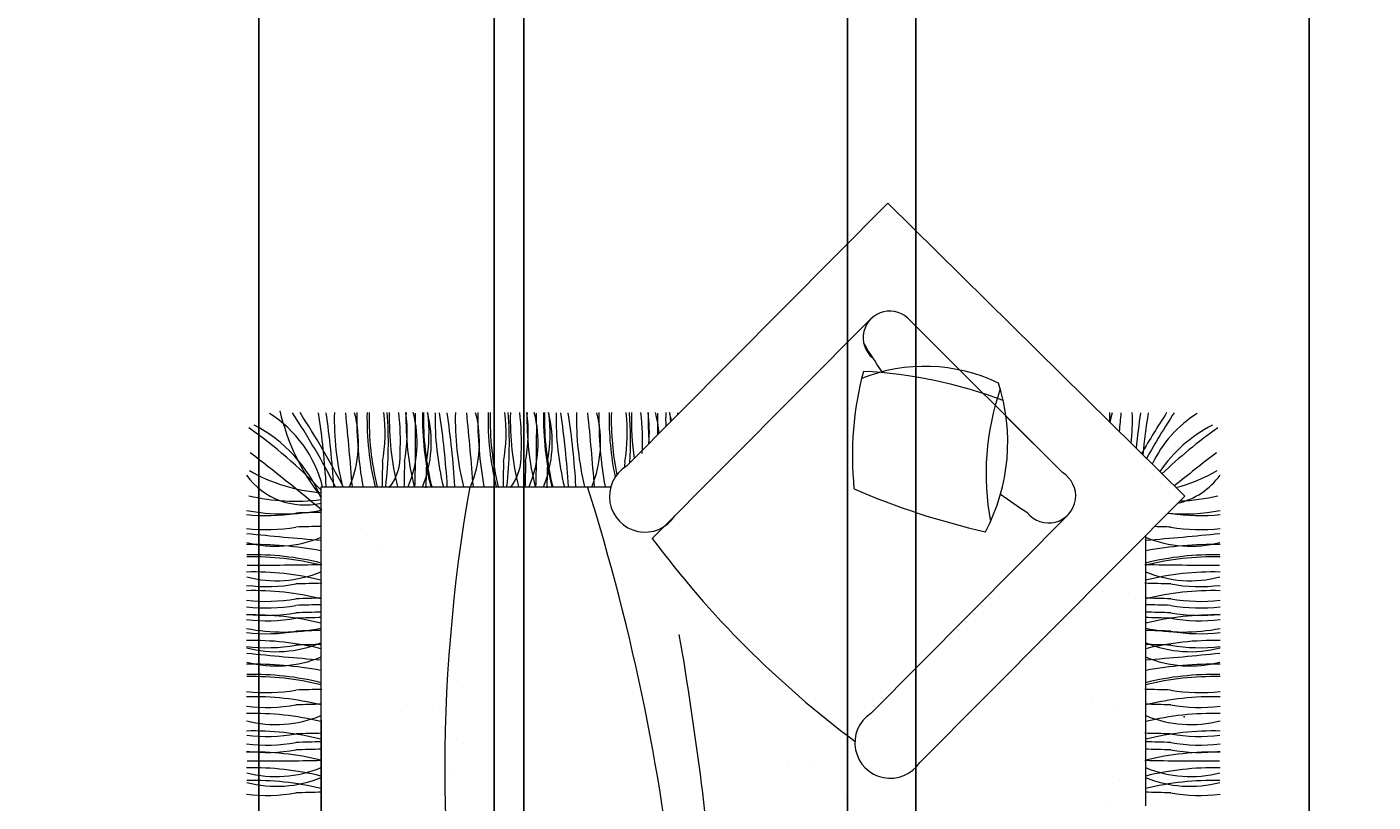
# Model space of a CAD drawing. Units: inches. Extents: x 503 to 1084, y -605 to 132.
# Tile 10 of 14: x 882 to 974, y -230 to -177. Entities that reach past the tile are written whole.
import ezdxf

# ---------------------------------------------------------------- set-up
doc = ezdxf.new("R2010")
doc.units = ezdxf.units.IN
doc.header["$MEASUREMENT"] = 0
doc.layers.add('A-ANNO-DIMS', color=7, linetype='Continuous', lineweight=18)
doc.layers.add('furniture', color=50, linetype='Continuous', lineweight=13, transparency=0.8)
doc.styles.get("Standard").update_dxf_attribs({"font": 'arial.ttf'})
doc.dimstyles.get("Standard").update_dxf_attribs({"dimtxt": 0.18, "dimasz": 0.18, "dimexe": 0.18, "dimexo": 0.0625, "dimgap": 0.09, "dimtad": 0, "dimtih": 1, "dimtoh": 1, "dimdec": 1, "dimzin": 0, "dimdsep": 46, "dimlunit": 4, "dimtxsty": 'Standard', "dimcen": 0.09, "dimadec": 0, "dimazin": 0, "dimtfac": 1, "dimtdec": 1, "dimtofl": 0, "dimtmove": 0, "dimatfit": 3, "dimfxl": 1, "dimtolj": 1, "dimtzin": 0, "dimarcsym": 0})

# ---------------------------------------------------------------- blocks, each defined once
blk = doc.blocks.new('CUSHION-SCATTER')
for centre, radius, start, end in [((-0.355, -5.979), 11.599, 64.45006, 111.76991), ((17.467, -0.489), 22.747, 165.30685, 185.5663), ((-5.995, -25.402), 30.717, 69.08153, 87.27682), ((-7.72, 0.481), 12.999, 332.0126, 17.9429), ((21.395, -1.669), 17.594, 160.90051, 190.65125), ((14.361, 41.881), 48.668, 246.33709, 257.41765)]:
    blk.add_arc(centre, radius, start, end)
blk = doc.blocks.new('*D45')
at = {"layer": 'A-ANNO-DIMS', "color": 0, "lineweight": -2, "transparency": 16777216}
for p, q in [((844.089, -354.753), (844.089, 43.514)), ((844.269, 43.334), (879.759, 43.334)), ((915.909, 43.334), (880.418, 43.334)), ((916.089, -354.753), (916.089, 43.514))]:
    blk.add_line(p, q, dxfattribs=at)
at = {"layer": 'A-ANNO-DIMS', "color": 0, "transparency": 16777216}
for points in [[(844.269, 43.364), (844.269, 43.304), (844.089, 43.334)], [(915.909, 43.364), (915.909, 43.304), (916.089, 43.334)]]:
    blk.add_solid(points, dxfattribs=at)
at = {"layer": 'Defpoints', "color": 0, "transparency": 16777216}
for p in [(916.089, 43.334), (844.089, -354.816), (916.089, -354.816)]:
    blk.add_point(p, dxfattribs=at)
at = {"layer": 'A-ANNO-DIMS', "color": 0, "transparency": 16777216, "insert": (880.089, 43.334), "char_height": 0.18, "attachment_point": 5}
blk.add_mtext('\\A1;6\'-0"', dxfattribs=at)
blk = doc.blocks.new('*D64')
at = {"layer": 'A-ANNO-DIMS', "color": 0, "lineweight": -2, "transparency": 16777216}
for p, q in [((938.089, -162.878), (938.089, -583.146)), ((977.089, -162.878), (977.089, -583.146)), ((938.269, -582.966), (957.26, -582.966)), ((976.909, -582.966), (957.918, -582.966))]:
    blk.add_line(p, q, dxfattribs=at)
at = {"layer": 'A-ANNO-DIMS', "color": 0, "transparency": 16777216}
for points in [[(938.269, -582.936), (938.269, -582.996), (938.089, -582.966)], [(976.909, -582.936), (976.909, -582.996), (977.089, -582.966)]]:
    blk.add_solid(points, dxfattribs=at)
at = {"layer": 'Defpoints', "color": 0, "transparency": 16777216}
for p in [(938.089, -162.816), (977.089, -162.816), (977.089, -582.966)]:
    blk.add_point(p, dxfattribs=at)
at = {"layer": 'A-ANNO-DIMS', "color": 0, "transparency": 16777216, "insert": (957.589, -582.966), "char_height": 0.18, "attachment_point": 5}
blk.add_mtext('\\A1;3\'-3"', dxfattribs=at)
blk = doc.blocks.new('*D65')
at = {"layer": 'A-ANNO-DIMS', "color": 0, "lineweight": -2, "transparency": 16777216}
for p, q in [((898.089, -162.878), (898.089, -583.146)), ((914.089, -162.878), (914.089, -583.146)), ((898.269, -582.966), (905.768, -582.966)), ((913.909, -582.966), (906.409, -582.966))]:
    blk.add_line(p, q, dxfattribs=at)
at = {"layer": 'A-ANNO-DIMS', "color": 0, "transparency": 16777216}
for points in [[(898.269, -582.936), (898.269, -582.996), (898.089, -582.966)], [(913.909, -582.936), (913.909, -582.996), (914.089, -582.966)]]:
    blk.add_solid(points, dxfattribs=at)
at = {"layer": 'Defpoints', "color": 0, "transparency": 16777216}
for p in [(898.089, -162.816), (914.089, -162.816), (914.089, -582.966)]:
    blk.add_point(p, dxfattribs=at)
at = {"layer": 'A-ANNO-DIMS', "color": 0, "transparency": 16777216, "insert": (906.089, -582.966), "char_height": 0.18, "attachment_point": 5}
blk.add_mtext('\\A1;1\'-4"', dxfattribs=at)
blk = doc.blocks.new('*D71')
at = {"layer": 'A-ANNO-DIMS', "color": 0, "lineweight": -2, "transparency": 16777216}
for p, q in [((942.746, -236.149), (942.746, 43.514)), ((942.926, 43.334), (955.566, 43.334)), ((969.287, 43.334), (956.647, 43.334)), ((969.467, -235.109), (969.467, 43.514))]:
    blk.add_line(p, q, dxfattribs=at)
at = {"layer": 'A-ANNO-DIMS', "color": 0, "transparency": 16777216}
for points in [[(942.926, 43.364), (942.926, 43.304), (942.746, 43.334)], [(969.287, 43.364), (969.287, 43.304), (969.467, 43.334)]]:
    blk.add_solid(points, dxfattribs=at)
at = {"layer": 'Defpoints', "color": 0, "transparency": 16777216}
for p in [(969.467, 43.334), (969.467, -235.171), (942.746, -236.212)]:
    blk.add_point(p, dxfattribs=at)
at = {"layer": 'A-ANNO-DIMS', "color": 0, "transparency": 16777216, "insert": (956.106, 43.334), "char_height": 0.18, "attachment_point": 5}
blk.add_mtext('\\A1;2\'-2 1/2"', dxfattribs=at)

msp = doc.modelspace()

# ---------------------------------------------------------------- linework, layer by layer
at = {"layer": 'furniture'}
for p, q in [((940.842, -188.826), (923.073, -206.695)), ((961.008, -208.74), (940.842, -188.826)), ((924.828, -211.612), (939.689, -196.679)), ((952.695, -207.138), (942.35, -196.793)), ((945.712, -200.155), (942.35, -196.793)), ((952.695, -207.138), (948.869, -203.312)), ((909.841, -204.939), (909.841, -204.939)), ((909.88, -205.415), (909.88, -205.415)), ((918.065, -204.939), (918.065, -204.939)), ((918.104, -205.415), (918.104, -205.415)), ((902.315, -308.222), (902.315, -208.108)), ((902.315, -208.108), (922.005, -208.108)), ((961.008, -208.74), (943.01, -226.844)), ((900.735, -209.7), (900.735, -209.7)), ((900.735, -209.7), (900.735, -209.7)), ((900.735, -209.7), (900.735, -209.7)), ((953.063, -210.02), (939.67, -223.504)), ((959.933, -209.7), (959.933, -209.7)), ((959.933, -209.7), (959.933, -209.7)), ((959.933, -209.7), (959.933, -209.7)), ((901.032, -210.912), (901.032, -210.912)), ((901.032, -210.912), (901.032, -210.912)), ((901.032, -210.912), (901.032, -210.912)), ((905.046, -210.939), (905.046, -210.939)), ((959.636, -210.912), (959.636, -210.912)), ((959.636, -210.912), (959.636, -210.912)), ((959.636, -210.912), (959.636, -210.912)), ((958.353, -211.41), (958.353, -229.789)), ((906.12, -212.447), (906.12, -212.447)), ((958.875, -213.557), (958.875, -213.557)), ((958.875, -213.557), (958.875, -213.557)), ((955.388, -215.247), (955.388, -215.247)), ((957.16, -215.375), (957.16, -215.375)), ((959.301, -217.841), (959.301, -217.841)), ((958.677, -219.623), (958.677, -219.623)), ((911.581, -221.238), (911.581, -221.238)), ((911.581, -221.238), (911.581, -221.238)), ((908.094, -222.928), (908.094, -222.928)), ((909.866, -223.056), (909.866, -223.056)), ((954.682, -222.776), (954.682, -222.776)), ((956.203, -222.893), (956.203, -222.893)), ((902.315, -223.932), (902.315, -308.222)), ((958.383, -223.668), (958.383, -223.668)), ((961.321, -223.379), (961.321, -223.379)), ((912.007, -225.523), (912.007, -225.523)), ((937.593, -225.079), (937.593, -225.079)), ((937.593, -225.079), (937.593, -225.079)), ((934.106, -226.769), (934.106, -226.769)), ((960.596, -226.163), (960.596, -226.163)), ((911.383, -227.304), (911.383, -227.304)), ((935.878, -226.897), (935.878, -226.897)), ((956.6, -227.987), (956.6, -227.987)), ((960.798, -228.54), (960.798, -228.54)), ((938.019, -229.364), (938.019, -229.364)), ((955.877, -229.481), (955.877, -229.481))]:
    msp.add_line(p, q, dxfattribs=at)
for centre, radius, start, end in [((940.967, -197.957), 1.807, 40.10925, 229.89075), ((969.526, -180.121), 35.395, 211.08667, 214.72696), ((914.057, -199.591), 14.916, 192.95229, 218.0769), ((853.121, -233.97), 56.461, 27.26685, 33.17806), ((853.631, -233.957), 56.461, 27.26685, 33.17806), ((847.93, -211.294), 54.836, 3.36442, 8.62286), ((848.44, -211.281), 54.836, 3.36442, 8.62286), ((922.401, -203.504), 19.184, 178.63307, 193.85735), ((681.204, -225.711), 223.934, 4.51462, 5.80171), ((896.994, -205.077), 7.865, 337.30984, 14.86132), ((930.218, -203.485), 25.474, 179.01954, 190.40392), ((924.623, -203.513), 19.184, 178.63307, 193.85735), ((924.766, -203.513), 19.184, 178.63307, 193.85735), ((895.286, -204.416), 11.387, 349.93491, 6.88295), ((880.977, -205.084), 25.914, 353.37018, 4.50636), ((926.135, -203.508), 19.184, 178.63307, 193.85735), ((889.96, -205.04), 17.75, 357.44348, 6.44133), ((896.783, -204.411), 11.387, 349.93491, 6.88295), ((927.27, -203.499), 19.184, 178.63307, 193.85735), ((900.98, -205.061), 7.865, 337.30984, 14.86132), ((901.945, -205.074), 7.865, 337.30984, 14.86132), ((928.398, -203.511), 19.184, 178.63307, 193.85735), ((928.462, -203.501), 19.184, 178.63307, 193.85735), ((898.269, -204.421), 11.387, 349.93491, 6.88295), ((929.255, -203.519), 19.184, 178.63307, 193.85735), ((856.154, -211.294), 54.836, 3.36442, 8.62286), ((856.664, -211.281), 54.836, 3.36442, 8.62286), ((930.624, -203.504), 19.184, 178.63307, 193.85735), ((689.428, -225.711), 223.934, 4.51462, 5.80171), ((905.218, -205.077), 7.865, 337.30984, 14.86132), ((938.442, -203.485), 25.474, 179.01954, 190.40392), ((932.847, -203.513), 19.184, 178.63307, 193.85735), ((932.99, -203.513), 19.184, 178.63307, 193.85735), ((903.51, -204.416), 11.387, 349.93491, 6.88295), ((889.201, -205.084), 25.914, 353.37018, 4.50636), ((934.359, -203.508), 19.184, 178.63307, 193.85735), ((898.184, -205.04), 17.75, 357.44348, 6.44133), ((905.007, -204.411), 11.387, 349.93491, 6.88295), ((935.494, -203.499), 19.184, 178.63307, 193.85735), ((909.204, -205.061), 7.865, 337.30984, 14.86132), ((910.169, -205.074), 7.865, 337.30984, 14.86132), ((936.622, -203.511), 19.184, 178.63307, 193.85735), ((936.686, -203.501), 19.184, 178.63307, 193.85735), ((906.493, -204.421), 11.387, 349.93491, 6.88295), ((937.479, -203.519), 19.184, 178.63307, 193.85735), ((864.387, -211.294), 54.836, 3.36442, 8.62286), ((864.897, -211.281), 54.836, 3.36442, 8.62286), ((938.857, -203.504), 19.184, 178.63307, 193.85735), ((697.661, -225.711), 223.934, 4.51462, 5.80171), ((913.451, -205.077), 7.865, 337.30984, 14.86132), ((946.675, -203.485), 25.474, 179.01954, 190.40392), ((941.08, -203.513), 19.184, 178.63307, 191.83019), ((941.223, -203.513), 19.184, 178.63307, 191.35191), ((911.743, -204.416), 11.387, 349.93491, 6.88295), ((897.434, -205.084), 25.914, 356.96769, 4.50636), ((942.592, -203.508), 19.184, 178.63307, 187.97978), ((906.417, -205.04), 17.75, 357.44348, 6.44133), ((943.727, -203.499), 19.184, 178.63307, 184.92383), ((913.24, -204.411), 11.387, 356.24526, 6.88295), ((917.437, -205.061), 7.865, 4.27566, 14.86132), ((944.919, -203.501), 19.184, 178.63307, 181.52384), ((918.402, -205.074), 7.865, 10.65917, 14.86132), ((914.725, -204.421), 11.387, 3.81728, 6.88295), ((945.711, -203.519), 19.184, 178.63307, 179.10459), ((930.45, -203.485), 25.474, 359.47531, 0.98046), ((963.674, -205.077), 7.865, 165.13868, 170.07522), ((1179.464, -225.711), 223.934, 174.19829, 174.52363), ((938.268, -203.504), 19.184, 355.05376, 1.36693), ((1012.228, -211.281), 54.836, 171.37714, 173.92031), ((1007.037, -233.957), 56.461, 146.82194, 150.13556), ((1012.738, -211.294), 54.836, 171.37714, 174.38877), ((1007.547, -233.97), 56.461, 146.82194, 150.50261), ((893.328, -212.521), 9.701, 22.11811, 62.69671), ((894.389, -210.105), 8.279, 13.99349, 57.72877), ((744.513, -204.223), 164.233, 358.62796, 0.39341), ((752.737, -204.223), 164.233, 358.62796, 0.39341), ((760.97, -204.223), 164.233, 359.8849, 0.39341), ((966.279, -210.105), 8.279, 122.27123, 154.62744), ((967.34, -212.521), 9.701, 117.30329, 145.70162), ((877.858, -231.706), 33.837, 43.716, 54.68473), ((982.81, -231.706), 33.837, 125.31527, 133.64566), ((802.813, -328.985), 155.386, 50.15682, 52.45592), ((1057.855, -328.985), 155.386, 127.54408, 128.89007), ((1033.458, -210.42), 127.023, 178.18909, 178.97752), ((904.267, -206.022), 3.43, 321.65644, 3.17437), ((1034.954, -210.415), 127.023, 178.18909, 178.97752), ((1036.44, -210.426), 127.023, 178.18909, 178.97752), ((1041.682, -210.42), 127.023, 178.18909, 178.97752), ((912.491, -206.022), 3.43, 321.65644, 3.17437), ((1043.178, -210.415), 127.023, 178.18909, 178.97752), ((1044.664, -210.426), 127.023, 178.18909, 178.97752), ((924.337, -208.759), 2.421, 121.46934, 326.90762), ((1049.914, -210.42), 127.023, 178.18909, 178.3576), ((901.229, -204.437), 4.899, 215.90571, 282.80539), ((903.172, -197.026), 11.499, 240.13503, 265.72435), ((951.762, -208.721), 1.838, 217.67477, 59.51812), ((957.496, -197.026), 11.499, 284.67923, 299.86497), ((959.439, -204.437), 4.899, 282.97771, 324.09429), ((1020.854, -227.369), 110.128, 169.92753, 191.22459), ((779.545, -252.476), 147.711, 5.44209, 17.47988), ((900.593, -195.241), 13.836, 256.72146, 277.14908), ((969.526, -180.121), 35.395, 233.54543, 237.11437), ((960.075, -195.241), 13.836, 272.5322, 283.27854), ((898.614, -198.673), 11.387, 263.11705, 280.06509), ((899.741, -197.189), 12.757, 258.75453, 281.58879), ((904.618, -336.845), 127.023, 91.02248, 91.81091), ((960.927, -197.189), 12.757, 265.1756, 281.24547), ((962.054, -198.673), 11.387, 259.93491, 276.88295), ((898.612, -199.625), 11.387, 263.11705, 280.06509), ((919.918, 11.514), 223.934, 264.19829, 265.48538), ((904.616, -337.796), 127.023, 91.02248, 91.81091), ((940.751, 11.514), 223.934, 274.51462, 275.80171), ((956.052, -337.796), 127.023, 88.18909, 88.67093), ((962.057, -199.625), 11.387, 259.93491, 276.88295), ((897.692, -237.5), 25.474, 79.59608, 90.98046), ((899.284, -204.276), 7.865, 255.13868, 292.69016), ((978.573, -171.691), 66.949, 216.60494, 233.33873), ((961.384, -204.276), 7.865, 247.30984, 284.86132), ((962.976, -237.5), 25.474, 89.01954, 100.40392), ((897.72, -231.905), 19.184, 76.14265, 91.36693), ((897.72, -232.048), 19.184, 76.14265, 91.36693), ((962.948, -231.905), 19.184, 88.63307, 103.85735), ((962.949, -232.048), 19.184, 88.63307, 103.85735), ((897.718, -233.073), 19.184, 76.14265, 91.36693), ((899.28, -206.62), 7.865, 255.13868, 292.69016), ((898.43, -49.188), 164.233, 269.60659, 271.37204), ((962.238, -49.188), 164.233, 268.62796, 270.39341), ((961.388, -206.62), 7.865, 247.30984, 284.86132), ((962.95, -233.073), 19.184, 88.63307, 103.85735), ((898.623, -203.493), 11.387, 263.11705, 280.06509), ((904.627, -341.664), 127.023, 91.02248, 91.81091), ((956.041, -341.664), 127.023, 88.18909, 88.97752), ((962.045, -203.493), 11.387, 259.93491, 276.88295), ((898.62, -204.499), 11.387, 263.11705, 280.06509), ((897.715, -234.342), 19.184, 76.14265, 91.36693), ((904.624, -342.671), 127.023, 91.02248, 91.81091), ((956.044, -342.671), 127.023, 88.18909, 88.97752), ((962.953, -234.342), 19.184, 88.63307, 103.85735), ((962.048, -204.499), 11.387, 259.93491, 276.88295), ((898.617, -205.453), 11.387, 263.11705, 280.06509), ((898.619, -204.95), 11.387, 263.11705, 280.06509), ((904.622, -343.624), 127.023, 91.02248, 91.81091), ((904.623, -343.121), 127.023, 91.02248, 91.81091), ((956.045, -343.121), 127.023, 88.18909, 88.97752), ((956.047, -343.624), 127.023, 88.18909, 88.97752), ((962.049, -204.95), 11.387, 259.93491, 276.88295), ((962.051, -205.453), 11.387, 259.93491, 276.88295), ((898.616, -205.822), 11.387, 263.11705, 280.06509), ((897.71, -235.992), 19.184, 76.14265, 91.36693), ((899.741, -205.215), 12.757, 258.75453, 281.58879), ((904.621, -343.993), 127.023, 91.02248, 91.81091), ((956.048, -343.993), 127.023, 88.18909, 88.97752), ((962.958, -235.992), 19.184, 88.63307, 103.85735), ((960.927, -205.215), 12.757, 258.41121, 281.24547), ((962.052, -205.822), 11.387, 259.93491, 276.88295), ((897.706, -237.733), 19.184, 76.14265, 91.36693), ((898.614, -206.7), 11.387, 263.11705, 280.06509), ((904.618, -344.871), 127.023, 91.02248, 91.81091), ((701.097, -256.901), 228.874, 4.61959, 9.75131), ((956.05, -344.871), 127.023, 88.18909, 88.97752), ((962.963, -237.733), 19.184, 88.63307, 103.85735), ((962.054, -206.7), 11.387, 259.93491, 276.88295), ((898.612, -207.651), 11.387, 263.11705, 280.06509), ((899.267, -211.443), 7.865, 255.13868, 292.69016), ((919.918, 3.377), 223.934, 264.19829, 265.48538), ((904.616, -345.822), 127.023, 91.02248, 91.81091), ((956.052, -345.822), 127.023, 88.18909, 88.97752), ((961.401, -211.443), 7.865, 247.30984, 284.86132), ((940.751, 3.377), 223.934, 274.51462, 275.80171), ((962.057, -207.651), 11.387, 259.93491, 276.88295), ((897.692, -245.637), 25.474, 79.59608, 90.98046), ((899.284, -212.413), 7.865, 255.13868, 292.69016), ((961.384, -212.413), 7.865, 247.30984, 284.86132), ((962.976, -245.637), 25.474, 89.01954, 100.40392), ((897.72, -240.042), 19.184, 76.14265, 91.36693), ((897.72, -240.185), 19.184, 76.14265, 91.36693), ((962.948, -240.042), 19.184, 88.63307, 103.85735), ((962.949, -240.185), 19.184, 88.63307, 103.85735), ((898.623, -210.705), 11.387, 263.11705, 280.06509), ((904.627, -348.877), 127.023, 91.02248, 91.81091), ((956.041, -348.877), 127.023, 88.18909, 88.97752), ((962.045, -210.705), 11.387, 259.93491, 276.88295), ((898.62, -211.712), 11.387, 263.11705, 280.06509), ((897.715, -241.554), 19.184, 76.14265, 91.36693), ((904.624, -349.883), 127.023, 91.02248, 91.81091), ((956.044, -349.883), 127.023, 88.18909, 88.97752), ((962.953, -241.554), 19.184, 88.63307, 103.85735), ((962.048, -211.712), 11.387, 259.93491, 276.88295), ((897.706, -242.689), 19.184, 76.14265, 91.36693), ((899.267, -216.399), 7.865, 255.13868, 292.69016), ((941.004, -225.51), 2.408, 123.6335, 326.3665), ((961.401, -216.399), 7.865, 247.30984, 284.86132), ((962.963, -242.689), 19.184, 88.63307, 103.85735), ((897.708, -243.881), 19.184, 76.14265, 91.36693), ((898.628, -213.688), 11.387, 263.11705, 280.06509), ((904.632, -351.859), 127.023, 91.02248, 91.81091), ((956.036, -351.859), 127.023, 88.18909, 88.97752), ((962.96, -243.881), 19.184, 88.63307, 103.85735), ((962.04, -213.688), 11.387, 259.93491, 276.88295), ((898.619, -214.271), 11.387, 263.11705, 280.06509), ((904.622, -352.945), 127.023, 91.02248, 91.81091), ((904.623, -352.442), 127.023, 91.02248, 91.81091), ((956.045, -352.442), 127.023, 88.18909, 88.97752), ((956.047, -352.945), 127.023, 88.18909, 88.97752), ((962.049, -214.271), 11.387, 259.93491, 276.88295), ((898.617, -214.773), 11.387, 263.11705, 280.06509), ((897.71, -245.312), 19.184, 76.14265, 91.36693), ((898.43, -62.504), 164.233, 269.60659, 271.37204), ((962.238, -62.504), 164.233, 268.62796, 270.39341), ((962.958, -245.312), 19.184, 88.63307, 103.85735), ((962.051, -214.773), 11.387, 259.93491, 276.88295), ((897.718, -246.388), 19.184, 76.14265, 91.36693), ((899.28, -219.935), 7.865, 255.13868, 292.69016), ((961.388, -219.935), 7.865, 247.30984, 284.86132), ((962.95, -246.388), 19.184, 88.63307, 103.85735), ((897.725, -247.245), 19.184, 76.14265, 91.36693), ((899.288, -220.596), 7.865, 255.13868, 292.69016), ((961.38, -220.596), 7.865, 247.30984, 284.86132), ((962.943, -247.245), 19.184, 88.63307, 103.85735), ((898.616, -217.695), 11.387, 263.11705, 280.06509), ((904.621, -355.866), 127.023, 91.02248, 91.81091), ((956.048, -355.866), 127.023, 88.18909, 88.97752), ((962.052, -217.695), 11.387, 259.93491, 276.88295)]:
    msp.add_arc(centre, radius, start, end, dxfattribs=at)
msp.add_point((960.972, -223.727), dxfattribs=at)

# ---------------------------------------------------------------- block references
msp.add_blockref('CUSHION-SCATTER', (943.707, -205.532), dxfattribs=at)

# ---------------------------------------------------------------- dimensions: what is measured, and where the dimension line sits
at = {"layer": 'A-ANNO-DIMS'}
for base, p1, p2, picture, middle in [((916.089, 43.334), (844.089, -354.816), (916.089, -354.816), '*D45', (880.089, 43.334)), ((969.467, 43.334), (942.746, -236.212), (969.467, -235.171), '*D71', (956.106, 43.334)), ((914.089, -582.966), (898.089, -162.816), (914.089, -162.816), '*D65', (906.089, -582.966)), ((977.089, -582.966), (938.089, -162.816), (977.089, -162.816), '*D64', (957.589, -582.966))]:
    dim = msp.add_linear_dim(base=base, p1=p1, p2=p2, dimstyle='Standard', override={"dimdec": 1, "dimlfac": 1, "dimrnd": 0, "dimzin": 1, "dimdsep": 46, "dimlunit": 4, "dimfrac": 2}, dxfattribs=at)
    dim.commit()
    dim.dimension.update_dxf_attribs({"geometry": picture, "text_midpoint": middle})

doc.saveas('drawing.dxf')
